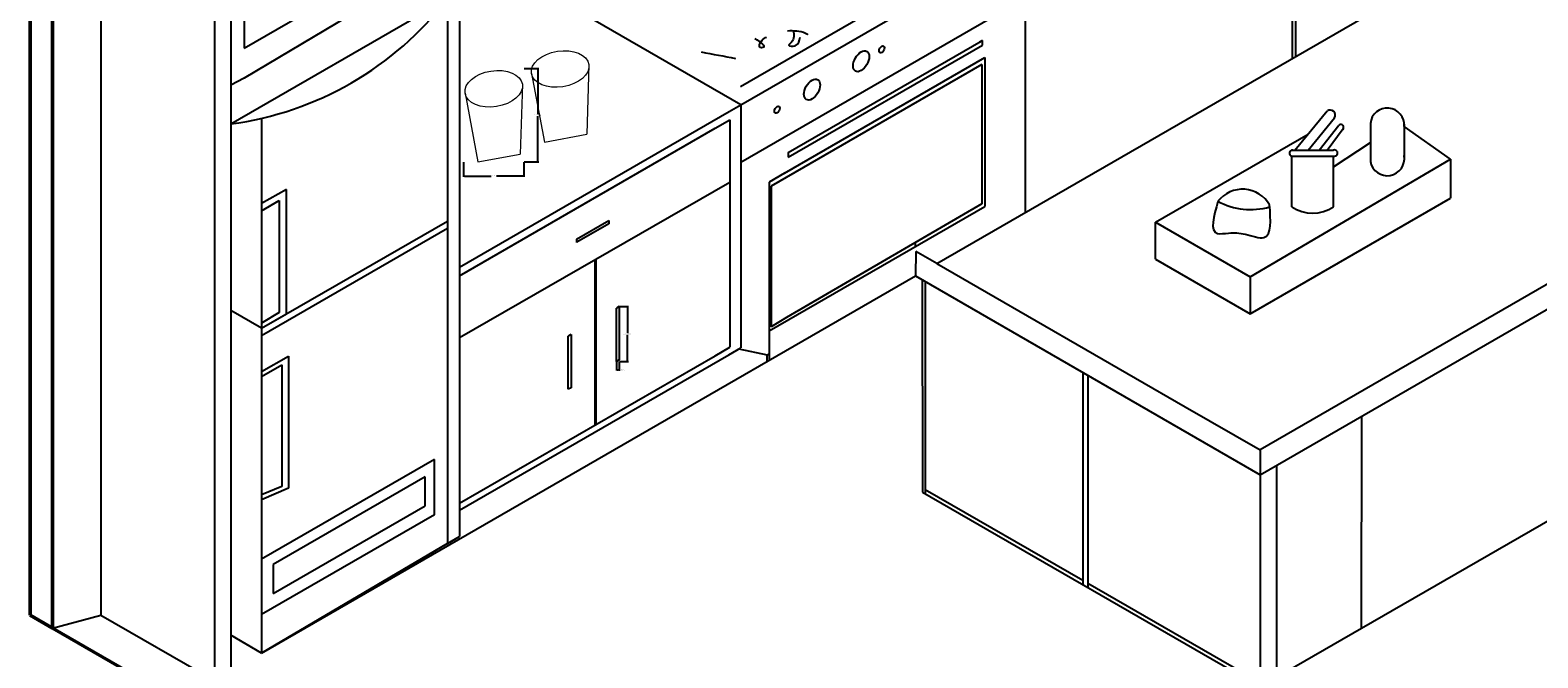
# Model space of a CAD drawing. Units: centimetres. Extents: x 5383 to 11288, y 5305 to 11515.
# Tile 2 of 5: x 5383 to 5675, y 5488 to 5610. Entities that reach past the tile are written whole.
import ezdxf

# ---------------------------------------------------------------- set-up
doc = ezdxf.new("R2010")
doc.units = ezdxf.units.CM
for name, color, linetype, lineweight in [('A-ANNO-DIMS', 2, 'Continuous', 18), ('A-EQPM', 4, 'Continuous', 25), ('A-FLOR-CASE', 3, 'Continuous', 25), ('A-FURN-ACCS', 9, 'Continuous', 13), ('A-WALL', 7, 'Continuous', 50)]:
    doc.layers.add(name, color=color, linetype=linetype, lineweight=lineweight)
doc.styles.get("Standard").update_dxf_attribs({"font": 'arial.ttf'})
doc.dimstyles.get("Standard").update_dxf_attribs({"dimtxt": 0.18, "dimasz": 0.18, "dimexe": 0.18, "dimexo": 0.0625, "dimgap": 0.09, "dimtad": 0, "dimtih": 1, "dimtoh": 1, "dimdec": 4, "dimzin": 0, "dimdsep": 46, "dimtxsty": 'Standard', "dimcen": 0.09, "dimadec": 0, "dimazin": 0, "dimtfac": 1, "dimtdec": 4, "dimtofl": 0, "dimtmove": 0, "dimatfit": 3, "dimfxl": 1, "dimtolj": 1, "dimtzin": 0, "dimarcsym": 0})

# ---------------------------------------------------------------- blocks, each defined once
blk = doc.blocks.new('HANDLE-DOOR-E')
for p, q in [((0.56, 10.64), (0, 10.32)), ((0, 0), (0, 10.32)), ((0.56, 10.64), (0.56, 0.32)), ((0.56, 0.32), (0, 0))]:
    blk.add_line(p, q)
blk = doc.blocks.new('CUP')
for p, q in [((11.09, 15.06), (10.7, 1.54)), ((0, 13.31), (2.49, 0)), ((2.49, 0), (10.7, 1.54))]:
    blk.add_line(p, q)
blk.add_ellipse((5.55, 14.18), major_axis=(-5.55, -0.87), ratio=0.619734)
blk = doc.blocks.new('*D14')
at = {"layer": 'A-ANNO-DIMS', "color": 0, "lineweight": -2, "transparency": 16777216}
for p, q in [((5478.47, 5602.2), (5481.3, 5602.2)), ((5481.12, 5602.02), (5481.12, 5593.33)), ((5481.12, 5584.28), (5481.12, 5592.97)), ((5478.47, 5584.1), (5481.3, 5584.1))]:
    blk.add_line(p, q, dxfattribs=at)
at = {"layer": 'A-ANNO-DIMS', "color": 0, "transparency": 16777216}
for points in [[(5481.09, 5602.02), (5481.15, 5602.02), (5481.12, 5602.2)], [(5481.09, 5584.28), (5481.15, 5584.28), (5481.12, 5584.1)]]:
    blk.add_solid(points, dxfattribs=at)
at = {"layer": 'Defpoints', "color": 0, "transparency": 16777216}
for p in [(5478.4, 5602.2), (5481.12, 5602.2), (5478.4, 5584.1)]:
    blk.add_point(p, dxfattribs=at)
at = {"layer": 'A-ANNO-DIMS', "color": 0, "transparency": 16777216, "insert": (5481.12, 5593.15), "char_height": 0.18, "attachment_point": 5}
blk.add_mtext('\\A1;CUP 18 TYP.', dxfattribs=at)
blk = doc.blocks.new('*D15')
at = {"layer": 'A-ANNO-DIMS', "color": 0, "lineweight": -2, "transparency": 16777216}
for p, q in [((5466.71, 5584.04), (5466.71, 5581.2)), ((5478.4, 5584.04), (5478.4, 5581.2)), ((5466.89, 5581.38), (5472.04, 5581.38)), ((5478.22, 5581.38), (5473.08, 5581.38))]:
    blk.add_line(p, q, dxfattribs=at)
at = {"layer": 'A-ANNO-DIMS', "color": 0, "transparency": 16777216}
for points in [[(5466.89, 5581.41), (5466.89, 5581.35), (5466.71, 5581.38)], [(5478.22, 5581.41), (5478.22, 5581.35), (5478.4, 5581.38)]]:
    blk.add_solid(points, dxfattribs=at)
at = {"layer": 'Defpoints', "color": 0, "transparency": 16777216}
for p in [(5466.71, 5584.1), (5478.4, 5584.1), (5478.4, 5581.38)]:
    blk.add_point(p, dxfattribs=at)
at = {"layer": 'A-ANNO-DIMS', "color": 0, "transparency": 16777216, "insert": (5472.56, 5581.38), "char_height": 0.18, "attachment_point": 5}
blk.add_mtext('\\A1;12 TYP.', dxfattribs=at)
blk = doc.blocks.new('*D28')
at = {"layer": 'A-ANNO-DIMS', "color": 0, "lineweight": -2, "transparency": 16777216}
for p, q in [((5496.92, 5556.1), (5498.63, 5556.1)), ((5498.45, 5555.92), (5498.45, 5550.96)), ((5498.45, 5545.64), (5498.45, 5550.6)), ((5496.92, 5545.46), (5498.63, 5545.46))]:
    blk.add_line(p, q, dxfattribs=at)
at = {"layer": 'A-ANNO-DIMS', "color": 0, "transparency": 16777216}
for points in [[(5498.42, 5555.92), (5498.48, 5555.92), (5498.45, 5556.1)], [(5498.42, 5545.64), (5498.48, 5545.64), (5498.45, 5545.46)]]:
    blk.add_solid(points, dxfattribs=at)
at = {"layer": 'Defpoints', "color": 0, "transparency": 16777216}
for p in [(5496.86, 5556.1), (5498.45, 5556.1), (5496.86, 5545.46)]:
    blk.add_point(p, dxfattribs=at)
at = {"layer": 'A-ANNO-DIMS', "color": 0, "transparency": 16777216, "insert": (5498.45, 5550.78), "char_height": 0.18, "attachment_point": 5}
blk.add_mtext('\\A1;HANDLE E 11 TYP.', dxfattribs=at)
blk = doc.blocks.new('*D29')
at = {"layer": 'A-ANNO-DIMS', "color": 0, "lineweight": -2, "transparency": 16777216}
for p, q in [((5496.3, 5545.4), (5496.3, 5543.69)), ((5496.86, 5545.4), (5496.86, 5543.69)), ((5496.48, 5543.87), (5496.68, 5543.87)), ((5496.86, 5543.87), (5497.04, 5543.87))]:
    blk.add_line(p, q, dxfattribs=at)
at = {"layer": 'A-ANNO-DIMS', "color": 0, "transparency": 16777216}
for points in [[(5496.48, 5543.9), (5496.48, 5543.84), (5496.3, 5543.87)], [(5496.68, 5543.9), (5496.68, 5543.84), (5496.86, 5543.87)]]:
    blk.add_solid(points, dxfattribs=at)
at = {"layer": 'Defpoints', "color": 0, "transparency": 16777216}
for p in [(5496.3, 5545.46), (5496.86, 5545.46), (5496.86, 5543.87)]:
    blk.add_point(p, dxfattribs=at)
at = {"layer": 'A-ANNO-DIMS', "color": 0, "transparency": 16777216, "insert": (5497.49, 5543.87), "char_height": 0.18, "attachment_point": 5}
blk.add_mtext('\\A1;1 TYP.', dxfattribs=at)

msp = doc.modelspace()

# ---------------------------------------------------------------- linework, layer by layer
at = {"layer": 'A-EQPM'}
for p, q in [((5424.24, 5635.93), (5424.24, 5606.15)), ((5424.24, 5606.15), (5461.66, 5627.75)), ((5520.4, 5595.18), (5575.44, 5626.96)), ((5465.93, 5625.19), (5424.24, 5600.32)), ((5520.3, 5598.74), (5567.93, 5626.24)), ((5575.44, 5615.8), (5520.4, 5584.02)), ((5575.44, 5615.8), (5575.44, 5574.33)), ((5520.4, 5595.18), (5486.72, 5614.62)), ((5529.55, 5585.94), (5566.93, 5607.52)), ((5529.55, 5585.03), (5567.17, 5606.75)), ((5567.17, 5607.66), (5566.59, 5607.32)), ((5567.17, 5606.75), (5567.17, 5607.66)), ((5528.81, 5581.92), (5567.6, 5604.31)), ((5567.6, 5604.31), (5567.6, 5575.49)), ((5424.24, 5600.32), (5421.66, 5598.99)), ((5567.02, 5602.95), (5526.26, 5579.41)), ((5567.02, 5602.95), (5567.02, 5575.99)), ((5518.1, 5593.85), (5520.4, 5595.18)), ((5520.4, 5595.18), (5520.4, 5549.28)), ((5465.93, 5563.73), (5518.1, 5593.85)), ((5529.55, 5585.94), (5529.55, 5585.03)), ((5528.81, 5581.92), (5525.87, 5580.22)), ((5525.87, 5580.22), (5525.87, 5549.56)), ((5526.26, 5579.41), (5526.26, 5552.15)), ((5525.87, 5551.39), (5567.6, 5575.49)), ((5567.02, 5575.99), (5529.23, 5553.98)), ((5554.18, 5567.74), (5554.18, 5568.51)), ((5529.23, 5553.98), (5526.26, 5552.15)), ((5525.87, 5551.39), (5525.87, 5545.71)), ((5518.04, 5546.75), (5520.4, 5548.12)), ((5520.01, 5547.89), (5525.5, 5546.73)), ((5520.4, 5549.28), (5520.4, 5548.12)), ((5465.93, 5516.67), (5518.04, 5546.75)), ((5525.5, 5546.73), (5525.87, 5546.96)), ((5525.5, 5545.49), (5525.5, 5546.73))]:
    msp.add_line(p, q, dxfattribs=at)
for centre, major_axis in [((5547.66, 5605.91), (-0.368, -0.638)), ((5543.67, 5603.61), (-1.11, -1.92)), ((5534.17, 5598.12), (-1.11, -1.92)), ((5527.41, 5594.22), (-0.368, -0.638))]:
    msp.add_ellipse(centre, major_axis=major_axis, ratio=0.57735, dxfattribs=at)
for points, knots in [([(5529.41, 5609.53), (5530.62, 5609.55), (5532.04, 5609.57), (5533.22, 5608.9), (5533.39, 5608.8)], [0, 0, 0, 0, 3.512962, 4.077974, 4.077974, 4.077974, 4.077974]), ([(5530.52, 5609.54), (5530.67, 5608.76), (5530.87, 5607.7), (5529.19, 5606.5), (5531.57, 5606.43), (5531.75, 5607.57), (5531.86, 5608.27)], [0, 0, 0, 0, 2.243303, 3.056707, 4.283829, 6.186562, 6.186562, 6.186562, 6.186562]), ([(5523.13, 5608.03), (5524.23, 5607.24), (5525.55, 5606.28), (5523.44, 5606.16), (5524.51, 5607.99), (5525.25, 5608.23), (5525.39, 5608.27)], [0, 0, 0, 0, 2.334899, 2.822963, 4.816434, 5.280999, 5.280999, 5.280999, 5.280999])]:
    msp.add_open_spline(points, degree=3, knots=knots, dxfattribs=at)
msp.add_open_spline([(5512.72, 5605.43), (5514.94, 5605), (5517.15, 5604.58), (5519.37, 5604.15)], degree=3, dxfattribs=at)
at = {"layer": 'A-FLOR-CASE'}
for p, q in [((5396.53, 5681.06), (5396.53, 5496.36)), ((5418.53, 5668.36), (5418.53, 5504.61)), ((5465.93, 5664.66), (5465.93, 5511.54)), ((5627.11, 5651.21), (5627.11, 5604.16)), ((5627.78, 5651.6), (5627.78, 5604.55)), ((5421.66, 5639.1), (5421.66, 5485.47)), ((5558.33, 5564.45), (5673.95, 5631.2)), ((5463.6, 5615.69), (5463.6, 5518.14)), ((5421.66, 5591.48), (5461.72, 5614.61)), ((5736.51, 5595.08), (5620.89, 5528.33)), ((5427.64, 5592.57), (5427.64, 5551.9)), ((5515.41, 5590.62), (5518.26, 5592.26)), ((5518.26, 5592.26), (5518.26, 5548.22)), ((5627.64, 5586.37), (5633.91, 5594.02)), ((5630.19, 5586.38), (5635.33, 5592.64)), ((5642.24, 5591.57), (5642.24, 5584.17)), ((5648.78, 5591.44), (5648.78, 5591.64)), ((5648.78, 5591.44), (5648.78, 5584.6)), ((5465.93, 5562.05), (5515.41, 5590.62)), ((5600.67, 5572.45), (5630.21, 5589.51)), ((5620.89, 5523.54), (5736.51, 5590.29)), ((5632.35, 5586.39), (5636.16, 5591.24)), ((5633.88, 5586.4), (5637, 5590.56)), ((5657.75, 5584.63), (5648.78, 5590.99)), ((5627.01, 5586.37), (5635.09, 5586.41)), ((5635.13, 5583.17), (5642.24, 5587.87)), ((5618.98, 5561.88), (5657.75, 5584.63)), ((5627.01, 5575.44), (5627.01, 5585.25)), ((5627.01, 5585.25), (5635.13, 5585.25)), ((5635.13, 5575.44), (5635.13, 5585.25)), ((5657.75, 5584.63), (5657.75, 5577.07)), ((5465.93, 5550.11), (5518.26, 5580.2)), ((5432.44, 5578.8), (5427.64, 5576.04)), ((5432.44, 5554.67), (5432.44, 5578.8)), ((5618.98, 5554.69), (5657.75, 5577.07)), ((5427.64, 5574.66), (5431.05, 5576.63)), ((5431.05, 5576.63), (5431.05, 5554.97)), ((5427.64, 5551.9), (5463.6, 5572.67)), ((5463.6, 5571.22), (5427.64, 5550.46)), ((5463.6, 5571.88), (5463.6, 5571.22)), ((5488.56, 5569.15), (5494.82, 5572.77)), ((5494.82, 5572.13), (5488.67, 5568.58)), ((5494.82, 5572.77), (5494.82, 5572.13)), ((5600.67, 5565.26), (5600.67, 5572.45)), ((5600.67, 5572.45), (5618.98, 5561.88)), ((5488.56, 5569.15), (5488.56, 5568.51)), ((5488.67, 5568.58), (5488.56, 5568.51)), ((5492.1, 5565.15), (5492.1, 5533.11)), ((5492.31, 5565.28), (5492.31, 5533.24)), ((5554.28, 5566.78), (5554.18, 5562.05)), ((5558.33, 5564.45), (5554.28, 5566.78)), ((5600.67, 5565.26), (5618.98, 5554.69)), ((5558.33, 5564.45), (5606.38, 5536.7)), ((5427.64, 5489), (5554.18, 5562.05)), ((5554.18, 5562.05), (5620.89, 5523.54)), ((5555.48, 5561.3), (5555.55, 5520.18)), ((5556.1, 5560.94), (5556.1, 5519.87)), ((5618.98, 5561.88), (5618.98, 5554.69)), ((5427.64, 5551.9), (5421.66, 5555.36)), ((5431.05, 5554.97), (5427.64, 5552.91)), ((5427.64, 5551.9), (5432.44, 5554.67)), ((5427.64, 5551.9), (5427.64, 5489)), ((5427.64, 5551.9), (5427.64, 5551.17)), ((5515.41, 5546.58), (5518.26, 5548.22)), ((5640.52, 5493.8), (5736.51, 5549.21)), ((5427.64, 5543.5), (5432.82, 5546.49)), ((5427.64, 5542.54), (5431.57, 5544.81)), ((5431.57, 5544.81), (5431.57, 5521.24)), ((5432.82, 5546.49), (5432.82, 5520.92)), ((5465.93, 5518.01), (5515.41, 5546.58)), ((5586.61, 5543.33), (5586.61, 5502.25)), ((5587.53, 5542.79), (5587.53, 5501.72)), ((5606.38, 5536.7), (5620.89, 5528.33)), ((5640.52, 5493.8), (5640.58, 5534.91)), ((5620.89, 5528.33), (5620.89, 5482.46)), ((5461.09, 5526.46), (5427.64, 5507.16)), ((5461.09, 5515.78), (5461.09, 5526.46)), ((5624.1, 5525.39), (5624.1, 5484.31)), ((5459.29, 5523.13), (5429.9, 5506.16)), ((5459.29, 5517.52), (5459.29, 5523.13)), ((5431.57, 5521.24), (5427.64, 5519.65)), ((5432.82, 5520.92), (5427.64, 5518.65)), ((5555.55, 5520.18), (5620.89, 5482.46)), ((5556.1, 5520.69), (5586.61, 5503.08)), ((5461.09, 5515.78), (5427.64, 5496.47)), ((5429.9, 5500.55), (5459.29, 5517.52)), ((5463.6, 5518.14), (5463.6, 5510.19)), ((5463.6, 5510.19), (5427.64, 5489)), ((5463.6, 5510.19), (5465.93, 5511.54)), ((5418.53, 5504.61), (5418.53, 5492.61)), ((5429.9, 5506.16), (5429.9, 5505.45)), ((5429.9, 5505.56), (5429.9, 5500.55)), ((5587.53, 5502.54), (5620.89, 5483.29)), ((5387.16, 5493.83), (5396.53, 5496.36)), ((5396.53, 5496.36), (5418.53, 5483.66)), ((5418.53, 5492.61), (5418.53, 5483.66)), ((5427.64, 5489), (5421.66, 5492.45)), ((5624.1, 5484.31), (5640.52, 5493.8))]:
    msp.add_line(p, q, dxfattribs=at)
for centre, radius, start, end in [((5413.21, 5654.54), 63.63, 277.6292, 322.3708), ((5645.51, 5591.28), 3.28, 354.9397, 174.9397), ((5634.43, 5593.13), 1.02, 331.4393, 120.259), ((5636.51, 5590.81), 0.554, 313.1572, 128.4295), ((5627.12, 5585.81), 0.571, 79.3497, 258.799), ((5635.28, 5585.83), 0.606, 255.2593, 109.0212), ((5645.51, 5584.76), 3.32, 190.2019, 10.2019), ((5617.5, 5572.79), 6.03, 29.6558, 142.2427), ((5619.12, 5588.44), 13.55, 241.8875, 285.6188), ((5631.07, 5581.47), 7.27, 236.0623, 303.9377)]:
    msp.add_arc(centre, radius, start, end, dxfattribs=at)
msp.add_open_spline([(5612.74, 5576.48), (5611.9, 5573.58), (5610.78, 5569.68), (5615.3, 5570.5), (5618, 5570.3), (5623.31, 5568.23), (5622.96, 5572.84), (5622.74, 5575.77)], degree=3, knots=[0, 0, 0, 0, 6.220698, 8.349484, 11.588439, 15.267112, 21.661902, 21.661902, 21.661902, 21.661902], dxfattribs=at)
at = {"layer": 'A-WALL'}
for p, q in [((5382.83, 5496.33), (5382.83, 5696.33)), ((5387.16, 5493.83), (5387.16, 5693.71)), ((5382.83, 5496.33), (5387.16, 5493.83)), ((5387.16, 5493.83), (5671.93, 5329.42))]:
    msp.add_line(p, q, dxfattribs=at)

# ---------------------------------------------------------------- block references
at = {"layer": 'A-FLOR-CASE'}
for p in [(5496.3, 5545.46), (5486.96, 5540.07)]:
    msp.add_blockref('HANDLE-DOOR-E', p, dxfattribs=at)
at = {"layer": 'A-FURN-ACCS'}
for p in [(5479.87, 5587.93), (5467.01, 5584.1)]:
    msp.add_blockref('CUP', p, dxfattribs=at)

# ---------------------------------------------------------------- dimensions: what is measured, and where the dimension line sits
at = {"layer": 'A-ANNO-DIMS'}
for base, p1, p2, text, picture, middle in [((5481.12, 5602.2), (5478.4, 5584.1), (5478.4, 5602.2), 'CUP <> TYP.', '*D14', (5481.12, 5593.15)), ((5498.45, 5556.1), (5496.86, 5545.46), (5496.86, 5556.1), 'HANDLE E <> TYP.', '*D28', (5498.45, 5550.78))]:
    dim = msp.add_linear_dim(base=base, p1=p1, p2=p2, angle=90, text=text, dimstyle='Standard', override={"dimdec": 0, "dimlfac": 1, "dimrnd": 0, "dimzin": 0, "dimdsep": 46, "dimlunit": 2}, dxfattribs=at)
    dim.commit()
    dim.dimension.update_dxf_attribs({"geometry": picture, "text_midpoint": middle})
for base, p1, p2, picture, middle in [((5478.4, 5581.38), (5466.71, 5584.1), (5478.4, 5584.1), '*D15', (5472.56, 5581.38)), ((5496.86, 5543.87), (5496.3, 5545.46), (5496.86, 5545.46), '*D29', (5497.49, 5543.87))]:
    dim = msp.add_linear_dim(base=base, p1=p1, p2=p2, text='<> TYP.', dimstyle='Standard', override={"dimdec": 0, "dimlfac": 1, "dimrnd": 0, "dimzin": 0, "dimdsep": 46, "dimlunit": 2}, dxfattribs=at)
    dim.commit()
    dim.dimension.update_dxf_attribs({"geometry": picture, "text_midpoint": middle})

doc.saveas('drawing.dxf')
